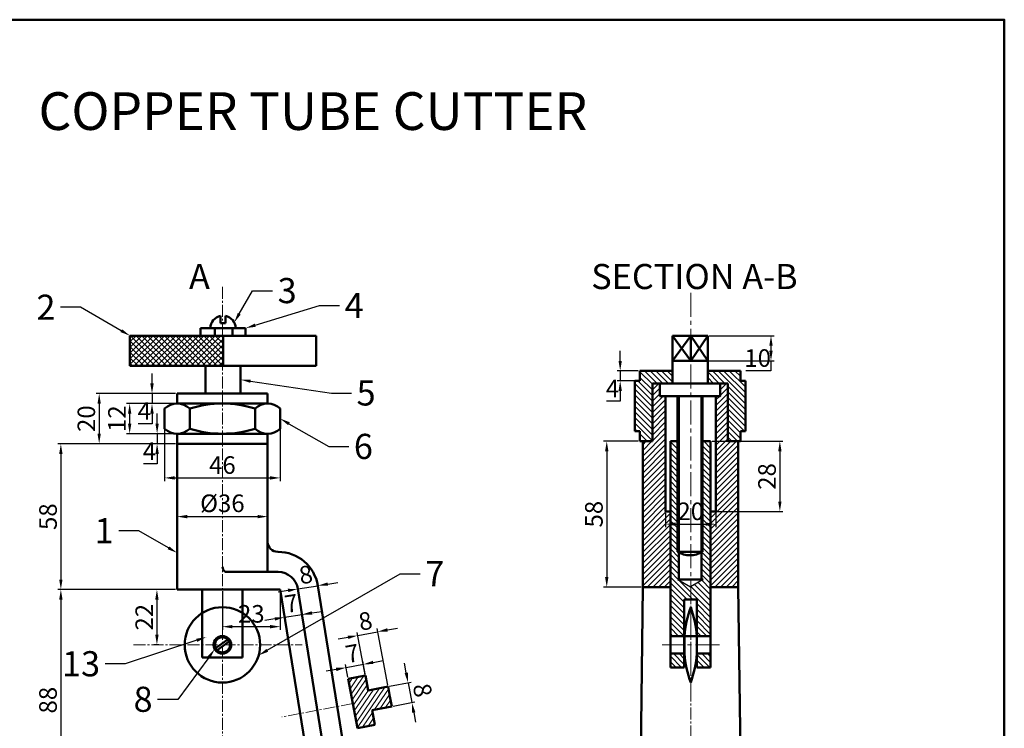
# Model space of a CAD drawing. Units: millimetres. Extents: x 376 to 1043, y -28 to 427.
# Tile 5 of 5: x 651 to 1043, y 145 to 427. Entities that reach past the tile are written whole.
import ezdxf
from ezdxf import colors
from ezdxf.entities.mleader import LeaderData, LeaderLine
from ezdxf.math import Vec2, Vec3

# ---------------------------------------------------------------- set-up
doc = ezdxf.new("R2010")
doc.units = ezdxf.units.MM
doc.header["$LTSCALE"] = 0.5
doc.linetypes.add('CENTER2', pattern=[28.575, 19.05, -3.175, 3.175, -3.175])
doc.linetypes.add('DASHED', pattern=[19.05, 12.7, -6.35])
for name, color, linetype, lineweight in [('M-CNTR', 1, 'CENTER2', 18), ('M-DIMS', 2, 'Continuous', 25), ('M-HATC', 8, 'Continuous', 18), ('M-HIDN', 4, 'DASHED', 25), ('M-OUTL', 7, 'Continuous', 50), ('M-TEXT', 7, 'Continuous', 25)]:
    doc.layers.add(name, color=color, linetype=linetype, lineweight=lineweight)
doc.styles.get("Standard").update_dxf_attribs({"font": 'arial.ttf'})
doc.dimstyles.new('ISO-25', dxfattribs={"dimtxt": 7, "dimasz": 4, "dimexe": 1.25, "dimexo": 0.625, "dimtad": 1, "dimtoh": 1, "dimtxsty": 'Standard', "dimcen": 2.5, "dimadec": 0, "dimazin": 0, "dimtfac": 1, "dimtmove": 0, "dimatfit": 3, "dimfxl": 1, "dimarcsym": 0})
pattern_1 = [(135, (1108.3857, -159.2338), (-1.122532, -1.122532), [])]

# ---------------------------------------------------------------- blocks, each defined once
blk = doc.blocks.new('*U20')
at = {"layer": 'M-CNTR', "color": 0, "transparency": 16777216}
blk.add_line((0, 74.83), (0, -77.3), dxfattribs=at)
blk = doc.blocks.new('*U26')
at = {"layer": 'M-CNTR', "color": 0, "transparency": 16777216}
blk.add_line((6.25, 0), (-16.57, 0), dxfattribs=at)
blk = doc.blocks.new('*D57')
at = {"layer": 'Defpoints', "color": 0, "ltscale": 0.5, "transparency": 16777216}
for p in [(713.94, 278.26), (703.95, 274.26), (713.94, 274.26)]:
    blk.add_point(p, dxfattribs=at)
at = {"layer": 'M-DIMS', "color": 0, "lineweight": -2, "ltscale": 0.5, "transparency": 16777216}
for p, q in [((703.95, 282.26), (703.95, 286.26)), ((713.32, 278.26), (702.7, 278.26)), ((703.95, 278.26), (703.95, 274.26)), ((713.32, 274.26), (702.7, 274.26)), ((703.95, 270.26), (703.95, 266.26)), ((703.95, 266.26), (698.48, 266.26))]:
    blk.add_line(p, q, dxfattribs=at)
at = {"layer": 'M-DIMS', "color": 0, "ltscale": 0.5, "transparency": 16777216}
for points in [[(703.28, 282.26), (704.62, 282.26), (703.95, 278.26)], [(703.28, 270.26), (704.62, 270.26), (703.95, 274.26)]]:
    blk.add_solid(points, dxfattribs=at)
at = {"layer": 'M-DIMS', "color": 0, "ltscale": 0.5, "transparency": 16777216, "insert": (700.9, 270.39), "char_height": 7, "attachment_point": 5}
blk.add_mtext('4', dxfattribs=at)
blk = doc.blocks.new('*D58')
at = {"layer": 'Defpoints', "color": 0, "ltscale": 0.5, "transparency": 16777216}
for p in [(713.94, 274.26), (695.06, 262.26), (713.94, 262.26)]:
    blk.add_point(p, dxfattribs=at)
at = {"layer": 'M-DIMS', "color": 0, "lineweight": -2, "ltscale": 0.5, "transparency": 16777216}
for p, q in [((713.32, 274.26), (693.81, 274.26)), ((695.06, 270.26), (695.06, 266.26)), ((713.32, 262.26), (693.81, 262.26))]:
    blk.add_line(p, q, dxfattribs=at)
at = {"layer": 'M-DIMS', "color": 0, "ltscale": 0.5, "transparency": 16777216}
for points in [[(694.4, 270.26), (695.73, 270.26), (695.06, 274.26)], [(694.4, 266.26), (695.73, 266.26), (695.06, 262.26)]]:
    blk.add_solid(points, dxfattribs=at)
at = {"layer": 'M-DIMS', "color": 0, "ltscale": 0.5, "transparency": 16777216, "insert": (690.92, 268.26), "char_height": 7, "attachment_point": 5, "rotation": 90}
blk.add_mtext('12', dxfattribs=at)
blk = doc.blocks.new('*D59')
at = {"layer": 'Defpoints', "color": 0, "ltscale": 0.5, "transparency": 16777216}
for p in [(713.94, 262.26), (705.98, 258.26), (713.94, 258.26)]:
    blk.add_point(p, dxfattribs=at)
at = {"layer": 'M-DIMS', "color": 0, "lineweight": -2, "ltscale": 0.5, "transparency": 16777216}
for p, q in [((705.98, 266.26), (705.98, 270.26)), ((713.32, 262.26), (704.73, 262.26)), ((705.98, 262.26), (705.98, 258.26)), ((713.32, 258.26), (704.73, 258.26)), ((705.98, 254.26), (705.98, 250.26)), ((705.98, 250.26), (700.52, 250.26))]:
    blk.add_line(p, q, dxfattribs=at)
at = {"layer": 'M-DIMS', "color": 0, "ltscale": 0.5, "transparency": 16777216}
for points in [[(705.32, 266.26), (706.65, 266.26), (705.98, 262.26)], [(705.32, 254.26), (706.65, 254.26), (705.98, 258.26)]]:
    blk.add_solid(points, dxfattribs=at)
at = {"layer": 'M-DIMS', "color": 0, "ltscale": 0.5, "transparency": 16777216, "insert": (702.94, 254.39), "char_height": 7, "attachment_point": 5}
blk.add_mtext('4', dxfattribs=at)
blk = doc.blocks.new('*D60')
at = {"layer": 'Defpoints', "color": 0, "ltscale": 0.5, "transparency": 16777216}
for p in [(713.94, 278.26), (682.94, 258.26), (713.94, 258.26)]:
    blk.add_point(p, dxfattribs=at)
at = {"layer": 'M-DIMS', "color": 0, "lineweight": -2, "ltscale": 0.5, "transparency": 16777216}
for p, q in [((713.32, 278.26), (681.69, 278.26)), ((682.94, 274.26), (682.94, 262.26)), ((713.32, 258.26), (681.69, 258.26))]:
    blk.add_line(p, q, dxfattribs=at)
at = {"layer": 'M-DIMS', "color": 0, "ltscale": 0.5, "transparency": 16777216}
for points in [[(682.27, 274.26), (683.6, 274.26), (682.94, 278.26)], [(682.27, 262.26), (683.6, 262.26), (682.94, 258.26)]]:
    blk.add_solid(points, dxfattribs=at)
at = {"layer": 'M-DIMS', "color": 0, "ltscale": 0.5, "transparency": 16777216, "insert": (678.74, 268.26), "char_height": 7, "attachment_point": 5, "rotation": 90}
blk.add_mtext('20', dxfattribs=at)
blk = doc.blocks.new('*D61')
at = {"layer": 'Defpoints', "color": 0, "ltscale": 0.5, "transparency": 16777216}
for p in [(697.5, 258.26), (667.7, 200.26), (713.94, 200.26)]:
    blk.add_point(p, dxfattribs=at)
at = {"layer": 'M-DIMS', "color": 0, "lineweight": -2, "ltscale": 0.5, "transparency": 16777216}
for p, q in [((696.88, 258.26), (666.45, 258.26)), ((667.7, 254.26), (667.7, 204.26)), ((713.32, 200.26), (666.45, 200.26))]:
    blk.add_line(p, q, dxfattribs=at)
at = {"layer": 'M-DIMS', "color": 0, "ltscale": 0.5, "transparency": 16777216}
for points in [[(667.03, 254.26), (668.37, 254.26), (667.7, 258.26)], [(667.03, 204.26), (668.37, 204.26), (667.7, 200.26)]]:
    blk.add_solid(points, dxfattribs=at)
at = {"layer": 'M-DIMS', "color": 0, "ltscale": 0.5, "transparency": 16777216, "insert": (663.5, 229.26), "char_height": 7, "attachment_point": 5, "rotation": 90}
blk.add_mtext('58', dxfattribs=at)
blk = doc.blocks.new('*D62')
at = {"layer": 'Defpoints', "color": 0, "ltscale": 0.5, "transparency": 16777216}
for p in [(707.25, 200.26), (705.91, 178.26), (707.25, 178.26)]:
    blk.add_point(p, dxfattribs=at)
at = {"layer": 'M-DIMS', "color": 0, "lineweight": -2, "ltscale": 0.5, "transparency": 16777216}
for p, q in [((706.63, 200.26), (704.66, 200.26)), ((705.91, 196.26), (705.91, 182.26)), ((706.63, 178.26), (704.66, 178.26))]:
    blk.add_line(p, q, dxfattribs=at)
at = {"layer": 'M-DIMS', "color": 0, "ltscale": 0.5, "transparency": 16777216}
for points in [[(705.24, 196.26), (706.57, 196.26), (705.91, 200.26)], [(705.24, 182.26), (706.57, 182.26), (705.91, 178.26)]]:
    blk.add_solid(points, dxfattribs=at)
at = {"layer": 'M-DIMS', "color": 0, "ltscale": 0.5, "transparency": 16777216, "insert": (701.77, 189.26), "char_height": 7, "attachment_point": 5, "rotation": 90}
blk.add_mtext('22', dxfattribs=at)
blk = doc.blocks.new('*D63')
at = {"layer": 'Defpoints', "color": 0, "ltscale": 0.5, "transparency": 16777216}
for p in [(689.88, 200.26), (667.7, 112.26), (689.88, 112.26)]:
    blk.add_point(p, dxfattribs=at)
at = {"layer": 'M-DIMS', "color": 0, "lineweight": -2, "ltscale": 0.5, "transparency": 16777216}
for p, q in [((689.26, 200.26), (666.45, 200.26)), ((667.7, 196.26), (667.7, 116.26)), ((689.26, 112.26), (666.45, 112.26))]:
    blk.add_line(p, q, dxfattribs=at)
at = {"layer": 'M-DIMS', "color": 0, "ltscale": 0.5, "transparency": 16777216}
for points in [[(667.03, 196.26), (668.37, 196.26), (667.7, 200.26)], [(667.03, 116.26), (668.37, 116.26), (667.7, 112.26)]]:
    blk.add_solid(points, dxfattribs=at)
at = {"layer": 'M-DIMS', "color": 0, "ltscale": 0.5, "transparency": 16777216, "insert": (663.5, 156.26), "char_height": 7, "attachment_point": 5, "rotation": 90}
blk.add_mtext('88', dxfattribs=at)
blk = doc.blocks.new('*D76')
at = {"layer": 'Defpoints', "color": 0, "ltscale": 0.5, "transparency": 16777216}
for p in [(756.71, 189.23), (763.62, 190.33), (763.62, 190.33)]:
    blk.add_point(p, dxfattribs=at)
at = {"layer": 'M-DIMS', "color": 0, "lineweight": -2, "ltscale": 0.5, "transparency": 16777216}
for p, q in [((752.76, 188.59), (748.81, 187.96)), ((756.61, 189.84), (756.51, 190.46)), ((756.71, 189.23), (763.62, 190.33)), ((763.53, 190.95), (763.43, 191.57)), ((767.57, 190.97), (771.52, 191.6))]:
    blk.add_line(p, q, dxfattribs=at)
at = {"layer": 'M-DIMS', "color": 0, "ltscale": 0.5, "transparency": 16777216}
for points in [[(752.66, 189.25), (752.87, 187.93), (756.71, 189.23)], [(767.47, 191.63), (767.68, 190.31), (763.62, 190.33)]]:
    blk.add_solid(points, dxfattribs=at)
at = {"layer": 'M-DIMS', "color": 0, "ltscale": 0.5, "transparency": 16777216, "insert": (759.52, 193.85), "char_height": 7, "attachment_point": 5, "rotation": 9.1114}
blk.add_mtext('7', dxfattribs=at)
blk = doc.blocks.new('*D77')
at = {"layer": 'Defpoints', "color": 0, "ltscale": 0.5, "transparency": 16777216}
for p in [(761.99, 200.53), (769.89, 201.8), (769.89, 201.8)]:
    blk.add_point(p, dxfattribs=at)
at = {"layer": 'M-DIMS', "color": 0, "lineweight": -2, "ltscale": 0.5, "transparency": 16777216}
for p, q in [((758.04, 199.9), (754.09, 199.26)), ((761.99, 200.53), (769.89, 201.8)), ((762.09, 199.91), (762.19, 199.3)), ((769.99, 201.18), (770.09, 200.56)), ((773.84, 202.43), (777.79, 203.06))]:
    blk.add_line(p, q, dxfattribs=at)
at = {"layer": 'M-DIMS', "color": 0, "ltscale": 0.5, "transparency": 16777216}
for points in [[(757.93, 200.56), (758.15, 199.24), (761.99, 200.53)], [(773.73, 203.09), (773.94, 201.77), (769.89, 201.8)]]:
    blk.add_solid(points, dxfattribs=at)
at = {"layer": 'M-DIMS', "color": 0, "ltscale": 0.5, "transparency": 16777216, "insert": (765.27, 205.31), "char_height": 7, "attachment_point": 5, "rotation": 9.1114}
blk.add_mtext('8', dxfattribs=at)
blk = doc.blocks.new('*D78')
at = {"layer": 'Defpoints', "color": 0, "ltscale": 0.5, "transparency": 16777216}
for p in [(731.94, 200.26), (754.94, 200.26), (731.94, 185.5)]:
    blk.add_point(p, dxfattribs=at)
at = {"layer": 'M-DIMS', "color": 0, "lineweight": -2, "ltscale": 0.5, "transparency": 16777216}
for p, q in [((731.94, 199.64), (731.94, 184.25)), ((754.94, 199.64), (754.94, 184.25)), ((750.94, 185.5), (735.94, 185.5))]:
    blk.add_line(p, q, dxfattribs=at)
at = {"layer": 'M-DIMS', "color": 0, "ltscale": 0.5, "transparency": 16777216}
for points in [[(735.94, 186.17), (735.94, 184.83), (731.94, 185.5)], [(750.94, 186.17), (750.94, 184.83), (754.94, 185.5)]]:
    blk.add_solid(points, dxfattribs=at)
at = {"layer": 'M-DIMS', "color": 0, "ltscale": 0.5, "transparency": 16777216, "insert": (743.44, 189.7), "char_height": 7, "attachment_point": 5}
blk.add_mtext('23', dxfattribs=at)
blk = doc.blocks.new('*D79')
at = {"layer": 'Defpoints', "color": 0, "ltscale": 0.5, "transparency": 16777216}
for p in [(713.94, 229.26), (749.94, 229.29), (749.94, 229.26)]:
    blk.add_point(p, dxfattribs=at)
at = {"layer": 'M-DIMS', "color": 0, "lineweight": -2, "ltscale": 0.5, "transparency": 16777216}
for p, q in [((713.94, 229.89), (713.94, 230.54)), ((717.94, 229.29), (745.94, 229.29)), ((749.94, 229.89), (749.94, 230.54))]:
    blk.add_line(p, q, dxfattribs=at)
at = {"layer": 'M-DIMS', "color": 0, "ltscale": 0.5, "transparency": 16777216}
for points in [[(717.94, 229.96), (717.94, 228.62), (713.94, 229.29)], [(745.94, 229.96), (745.94, 228.62), (749.94, 229.29)]]:
    blk.add_solid(points, dxfattribs=at)
at = {"layer": 'M-DIMS', "color": 0, "ltscale": 0.5, "transparency": 16777216, "insert": (731.94, 233.68), "char_height": 7, "attachment_point": 5}
blk.add_mtext('%%C36', dxfattribs=at)
blk = doc.blocks.new('*D80')
at = {"layer": 'Defpoints', "color": 0, "ltscale": 0.5, "transparency": 16777216}
for p in [(708.94, 268.26), (754.94, 268.26), (754.94, 244.69)]:
    blk.add_point(p, dxfattribs=at)
at = {"layer": 'M-DIMS', "color": 0, "lineweight": -2, "ltscale": 0.5, "transparency": 16777216}
for p, q in [((708.94, 267.64), (708.94, 243.44)), ((754.94, 267.64), (754.94, 243.44)), ((712.94, 244.69), (750.94, 244.69))]:
    blk.add_line(p, q, dxfattribs=at)
at = {"layer": 'M-DIMS', "color": 0, "ltscale": 0.5, "transparency": 16777216}
for points in [[(712.94, 245.35), (712.94, 244.02), (708.94, 244.69)], [(750.94, 245.35), (750.94, 244.02), (754.94, 244.69)]]:
    blk.add_solid(points, dxfattribs=at)
at = {"layer": 'M-DIMS', "color": 0, "ltscale": 0.5, "transparency": 16777216, "insert": (731.94, 248.89), "char_height": 7, "attachment_point": 5}
blk.add_mtext('46', dxfattribs=at)
blk = doc.blocks.new('*D82')
at = {"layer": 'Defpoints', "color": 0, "ltscale": 0.5, "transparency": 16777216}
for p in [(788, 170.53), (781.97, 164.76), (788.85, 166.07)]:
    blk.add_point(p, dxfattribs=at)
at = {"layer": 'M-DIMS', "color": 0, "lineweight": -2, "ltscale": 0.5, "transparency": 16777216}
for p, q in [((777.19, 168.49), (773.26, 167.74)), ((781.85, 165.38), (780.89, 170.46)), ((781.12, 169.23), (788, 170.53)), ((788.73, 166.68), (787.77, 171.76)), ((791.93, 171.28), (795.86, 172.02))]:
    blk.add_line(p, q, dxfattribs=at)
at = {"layer": 'M-DIMS', "color": 0, "ltscale": 0.5, "transparency": 16777216}
for points in [[(777.07, 169.14), (777.32, 167.83), (781.12, 169.23)], [(791.81, 171.93), (792.05, 170.62), (788, 170.53)]]:
    blk.add_solid(points, dxfattribs=at)
at = {"layer": 'M-DIMS', "color": 0, "ltscale": 0.5, "transparency": 16777216, "insert": (783.79, 173.94), "char_height": 7, "attachment_point": 5, "rotation": 10.7228}
blk.add_mtext('7', dxfattribs=at)
blk = doc.blocks.new('*D83')
at = {"layer": 'Defpoints', "color": 0, "ltscale": 0.5, "transparency": 16777216}
for p in [(793.69, 183.49), (797.82, 161.66), (789.96, 160.17)]:
    blk.add_point(p, dxfattribs=at)
at = {"layer": 'M-DIMS', "color": 0, "lineweight": -2, "ltscale": 0.5, "transparency": 16777216}
for p, q in [((797.71, 162.27), (793.46, 184.71)), ((797.62, 184.23), (801.55, 184.97)), ((781.9, 181.25), (777.97, 180.51)), ((789.85, 160.78), (785.6, 183.23)), ((785.83, 182), (793.69, 183.49))]:
    blk.add_line(p, q, dxfattribs=at)
at = {"layer": 'M-DIMS', "color": 0, "ltscale": 0.5, "transparency": 16777216}
for points in [[(797.49, 184.89), (797.74, 183.58), (793.69, 183.49)], [(781.77, 181.91), (782.02, 180.6), (785.83, 182)]]:
    blk.add_solid(points, dxfattribs=at)
at = {"layer": 'M-DIMS', "color": 0, "ltscale": 0.5, "transparency": 16777216, "insert": (788.98, 186.87), "char_height": 7, "attachment_point": 5, "rotation": 10.7228}
blk.add_mtext('8', dxfattribs=at)
blk = doc.blocks.new('*D84')
at = {"layer": 'Defpoints', "color": 0, "ltscale": 0.5, "transparency": 16777216}
for p in [(797.82, 161.66), (799.31, 153.8), (807.29, 155.31)]:
    blk.add_point(p, dxfattribs=at)
at = {"layer": 'M-DIMS', "color": 0, "lineweight": -2, "ltscale": 0.5, "transparency": 16777216}
for p, q in [((805.06, 167.1), (804.32, 171.03)), ((798.44, 161.77), (807.03, 163.4)), ((805.8, 163.17), (807.29, 155.31)), ((799.92, 153.91), (808.52, 155.54)), ((808.04, 151.38), (808.78, 147.45))]:
    blk.add_line(p, q, dxfattribs=at)
at = {"layer": 'M-DIMS', "color": 0, "ltscale": 0.5, "transparency": 16777216}
for points in [[(805.72, 167.22), (804.41, 166.98), (805.8, 163.17)], [(808.69, 151.5), (807.38, 151.26), (807.29, 155.31)]]:
    blk.add_solid(points, dxfattribs=at)
at = {"layer": 'M-DIMS', "color": 0, "ltscale": 0.5, "transparency": 16777216, "insert": (810.67, 160.02), "char_height": 7, "attachment_point": 5, "rotation": 280.7228}
blk.add_mtext('8', dxfattribs=at)
blk = doc.blocks.new('*D88')
at = {"layer": 'Defpoints', "color": 0, "ltscale": 0.5, "transparency": 16777216}
for p in [(908.2, 231.26), (928.2, 231.26), (928.2, 226.29)]:
    blk.add_point(p, dxfattribs=at)
at = {"layer": 'M-DIMS', "color": 0, "lineweight": -2, "ltscale": 0.5, "transparency": 16777216}
for p, q in [((908.2, 230.64), (908.2, 225.04)), ((928.2, 230.64), (928.2, 225.04)), ((912.2, 226.29), (924.2, 226.29))]:
    blk.add_line(p, q, dxfattribs=at)
at = {"layer": 'M-DIMS', "color": 0, "ltscale": 0.5, "transparency": 16777216}
for points in [[(912.2, 226.96), (912.2, 225.62), (908.2, 226.29)], [(924.2, 226.96), (924.2, 225.62), (928.2, 226.29)]]:
    blk.add_solid(points, dxfattribs=at)
at = {"layer": 'M-DIMS', "color": 0, "ltscale": 0.5, "transparency": 16777216, "insert": (918.2, 230.49), "char_height": 7, "attachment_point": 5}
blk.add_mtext('20', dxfattribs=at)
blk = doc.blocks.new('*D89')
at = {"layer": 'Defpoints', "color": 0, "ltscale": 0.5, "transparency": 16777216}
for p in [(897.95, 259.26), (884.8, 201.26), (899.11, 201.26)]:
    blk.add_point(p, dxfattribs=at)
at = {"layer": 'M-DIMS', "color": 0, "lineweight": -2, "ltscale": 0.5, "transparency": 16777216}
for p, q in [((897.32, 259.26), (883.55, 259.26)), ((884.8, 255.26), (884.8, 205.26)), ((898.48, 201.26), (883.55, 201.26))]:
    blk.add_line(p, q, dxfattribs=at)
at = {"layer": 'M-DIMS', "color": 0, "ltscale": 0.5, "transparency": 16777216}
for points in [[(884.13, 255.26), (885.47, 255.26), (884.8, 259.26)], [(884.13, 205.26), (885.47, 205.26), (884.8, 201.26)]]:
    blk.add_solid(points, dxfattribs=at)
at = {"layer": 'M-DIMS', "color": 0, "ltscale": 0.5, "transparency": 16777216, "insert": (880.6, 230.26), "char_height": 7, "attachment_point": 5, "rotation": 90}
blk.add_mtext('58', dxfattribs=at)
blk = doc.blocks.new('*D90')
at = {"layer": 'Defpoints', "color": 0, "ltscale": 0.5, "transparency": 16777216}
for p in [(924.95, 301.26), (924.95, 291.26), (950.12, 291.26)]:
    blk.add_point(p, dxfattribs=at)
at = {"layer": 'M-DIMS', "color": 0, "lineweight": -2, "ltscale": 0.5, "transparency": 16777216}
for p, q in [((925.57, 301.26), (951.37, 301.26)), ((950.12, 297.26), (950.12, 295.26)), ((925.57, 291.26), (951.37, 291.26)), ((950.12, 291.26), (950.12, 287.26)), ((950.12, 287.26), (940.15, 287.26))]:
    blk.add_line(p, q, dxfattribs=at)
at = {"layer": 'M-DIMS', "color": 0, "ltscale": 0.5, "transparency": 16777216}
for points in [[(949.46, 297.26), (950.79, 297.26), (950.12, 301.26)], [(949.46, 295.26), (950.79, 295.26), (950.12, 291.26)]]:
    blk.add_solid(points, dxfattribs=at)
at = {"layer": 'M-DIMS', "color": 0, "ltscale": 0.5, "transparency": 16777216, "insert": (944.83, 291.46), "char_height": 7, "attachment_point": 5}
blk.add_mtext('10', dxfattribs=at)
blk = doc.blocks.new('*D91')
at = {"layer": 'Defpoints', "color": 0, "ltscale": 0.5, "transparency": 16777216}
for p in [(926.11, 259.26), (926.11, 231.26), (953.65, 231.26)]:
    blk.add_point(p, dxfattribs=at)
at = {"layer": 'M-DIMS', "color": 0, "lineweight": -2, "ltscale": 0.5, "transparency": 16777216}
for p, q in [((926.73, 259.26), (954.9, 259.26)), ((953.65, 255.26), (953.65, 235.26)), ((926.73, 231.26), (954.9, 231.26))]:
    blk.add_line(p, q, dxfattribs=at)
at = {"layer": 'M-DIMS', "color": 0, "ltscale": 0.5, "transparency": 16777216}
for points in [[(952.99, 255.26), (954.32, 255.26), (953.65, 259.26)], [(952.99, 235.26), (954.32, 235.26), (953.65, 231.26)]]:
    blk.add_solid(points, dxfattribs=at)
at = {"layer": 'M-DIMS', "color": 0, "ltscale": 0.5, "transparency": 16777216, "insert": (949.45, 245.26), "char_height": 7, "attachment_point": 5, "rotation": 90}
blk.add_mtext('28', dxfattribs=at)
blk = doc.blocks.new('*D92')
at = {"layer": 'Defpoints', "color": 0, "ltscale": 0.5, "transparency": 16777216}
for p in [(897.95, 287.26), (890.15, 283.26), (897.95, 283.26)]:
    blk.add_point(p, dxfattribs=at)
at = {"layer": 'M-DIMS', "color": 0, "lineweight": -2, "ltscale": 0.5, "transparency": 16777216}
for p, q in [((890.15, 291.26), (890.15, 295.26)), ((897.32, 287.26), (888.9, 287.26)), ((890.15, 287.26), (890.15, 283.26)), ((897.32, 283.26), (888.9, 283.26)), ((890.15, 279.26), (890.15, 275.26)), ((890.15, 275.26), (884.69, 275.26))]:
    blk.add_line(p, q, dxfattribs=at)
at = {"layer": 'M-DIMS', "color": 0, "ltscale": 0.5, "transparency": 16777216}
for points in [[(889.49, 291.26), (890.82, 291.26), (890.15, 287.26)], [(889.49, 279.26), (890.82, 279.26), (890.15, 283.26)]]:
    blk.add_solid(points, dxfattribs=at)
at = {"layer": 'M-DIMS', "color": 0, "ltscale": 0.5, "transparency": 16777216, "insert": (887.11, 279.39), "char_height": 7, "attachment_point": 5}
blk.add_mtext('4', dxfattribs=at)

msp = doc.modelspace()

# ---------------------------------------------------------------- hatches: boundary and pattern name
at = {"layer": 'M-HATC', "ltscale": 0.5}
h = msp.add_hatch(dxfattribs=at)
h.set_pattern_fill('ANSI37', color=256, scale=0.5)
h.set_pattern_definition([(45, (907.5903, -133.1619), (-1.122532, 1.122532), []), (135, (907.5903, -133.1619), (-1.122532, -1.122532), [])])
h.paths.add_polyline_path([(732.193, 289.264), (732.193, 301.264), (695.193, 301.264), (695.193, 289.264)])
h = msp.add_hatch(dxfattribs=at)
h.set_pattern_fill('ANSI31', color=256, scale=0.5, angle=90)
h.set_pattern_definition(pattern_1)
h.paths.add_polyline_path([(902.946, 282.264), (905.946, 282.264), (910.946, 282.264), (910.946, 287.264), (897.946, 287.264), (897.946, 283.264), (895.946, 283.264), (895.946, 263.264), (897.946, 263.264), (897.946, 259.264), (902.946, 259.264)])
h.paths.add_polyline_path([(939.946, 283.264), (937.946, 283.264), (937.946, 287.264), (924.946, 287.264), (924.946, 282.264), (929.946, 282.264), (932.946, 282.264), (932.946, 273.535), (932.946, 259.264), (937.946, 259.264), (937.946, 263.264), (939.946, 263.264)])
h = msp.add_hatch(dxfattribs=at)
h.set_pattern_fill('ANSI31', color=256, scale=0.5)
h.set_pattern_definition([(45, (1108.3857, -159.2338), (-1.122532, 1.122532), [])])
h.paths.add_polyline_path([(899.107, 201.264), (910.107, 201.264), (910.107, 231.264), (908.196, 231.264), (908.196, 277.264), (905.946, 277.264), (905.946, 282.264), (902.946, 282.264), (902.946, 259.264), (899.107, 259.264)])
h.paths.add_polyline_path([(937.107, 259.264), (932.946, 259.264), (932.946, 273.535), (932.946, 282.264), (929.946, 282.264), (929.946, 277.264), (928.196, 277.264), (928.196, 231.264), (926.107, 231.264), (926.107, 201.264), (937.107, 201.264)])
h = msp.add_hatch(dxfattribs=at)
h.set_pattern_fill('ANSI31', color=256, scale=0.5, angle=90)
h.set_pattern_definition(pattern_1)
h.paths.add_polyline_path([(926.107, 259.264), (922.946, 259.264), (922.946, 215.264, -0.0142093), (922.446, 214.994), (922.446, 204.264), (923.107, 204.264), (918.107, 201.378), (913.107, 204.264), (913.446, 204.264), (913.446, 214.994, -0.0142093), (912.946, 215.264), (912.946, 259.264), (910.107, 259.264), (910.107, 181.764), (915.607, 181.764), (915.607, 196.264), (920.607, 196.264), (920.607, 182.699, -0.0051135), (920.696, 181.764), (926.107, 181.764)])
h = msp.add_hatch(dxfattribs=at)
h.set_pattern_fill('ANSI31', color=256, scale=0.5, angle=90)
h.set_pattern_definition(pattern_1)
h.paths.add_polyline_path([(915.607, 174.764), (910.107, 174.764), (910.107, 169.264), (915.607, 169.264)])
h.paths.add_polyline_path([(926.107, 174.764), (920.696, 174.764, -0.0051135), (920.607, 173.83), (920.607, 169.264), (926.107, 169.264)])
h = msp.add_hatch(dxfattribs=at)
h.set_pattern_fill('ANSI31', color=256, scale=0.5, angle=10.7228)
h.set_pattern_definition([(55.7228, (1132.0873, -118.6822), (-1.311787, 0.8940756), [])])
h.paths.add_polyline_path([(799.31, 153.798), (798.566, 157.728), (797.822, 161.659), (789.962, 160.17), (788.845, 166.065), (781.967, 164.763), (785.689, 145.112), (792.566, 146.415), (791.45, 152.31)])

# ---------------------------------------------------------------- linework, layer by layer
at = {"layer": 'M-CNTR', "ltscale": 0.5}
for p, q in [((731.943, 320.737), (731.943, -3.612)), ((918.196, 160.434), (918.196, 196.785)), ((696.645, 178.264), (763.736, 178.264)), ((918.196, 160.434), (918.196, 11.662)), ((783.828, 154.938), (755.538, 149.58))]:
    msp.add_line(p, q, dxfattribs=at)
at = {"layer": 'M-HIDN'}
for p, q in [((913.107, 215.264), (913.107, 215.174)), ((922.607, 215.264), (922.607, 215.077)), ((913.107, 204.264), (918.107, 201.378)), ((923.107, 204.264), (918.107, 201.378))]:
    msp.add_line(p, q, dxfattribs=at)
at = {"layer": 'M-OUTL'}
for p, q in [((731.193, 306.264), (731.193, 309.163)), ((732.193, 306.264), (731.193, 306.264)), ((732.193, 306.264), (733.193, 306.264)), ((733.193, 306.264), (733.193, 309.163)), ((741.193, 304.264), (723.193, 304.264)), ((723.193, 304.264), (723.193, 301.264)), ((727.193, 304.264), (737.193, 304.264)), ((728.935, 304.264), (728.935, 301.264)), ((735.998, 304.264), (735.998, 301.264)), ((741.193, 301.264), (741.193, 304.264)), ((769.193, 301.264), (695.193, 301.264)), ((695.193, 301.264), (695.193, 289.264)), ((723.193, 301.264), (741.193, 301.264)), ((732.193, 301.264), (732.193, 289.264)), ((769.193, 289.264), (769.193, 301.264)), ((910.946, 301.264), (924.946, 301.264)), ((910.946, 282.264), (910.946, 301.264)), ((924.946, 301.264), (924.946, 282.264)), ((695.193, 289.264), (769.193, 289.264)), ((713.943, 278.264), (724.943, 278.264)), ((713.943, 274.264), (713.943, 278.264)), ((724.943, 278.264), (738.943, 278.264)), ((738.943, 278.264), (749.943, 278.264)), ((749.943, 278.264), (749.943, 274.264)), ((749.943, 274.264), (713.943, 274.264)), ((912.946, 277.264), (912.946, 215.264)), ((913.446, 277.264), (913.446, 204.264)), ((922.446, 277.264), (922.446, 204.264)), ((922.946, 277.264), (922.946, 215.264)), ((910.107, 259.264), (912.946, 259.264)), ((910.107, 169.264), (910.107, 259.264)), ((922.946, 259.264), (926.107, 259.264)), ((926.107, 259.264), (926.107, 169.264)), ((912.946, 215.264), (922.946, 215.264)), ((915.607, 181.764), (910.107, 181.764)), ((926.107, 181.764), (920.607, 181.764)), ((915.607, 174.764), (910.107, 174.764)), ((926.107, 174.764), (920.607, 174.764)), ((915.607, 169.264), (910.107, 169.264)), ((926.107, 169.264), (920.607, 169.264))]:
    msp.add_line(p, q, dxfattribs=at)
at = {"layer": 'M-OUTL', "ltscale": 0.5}
for p, q in [((910.946, 301.264), (924.946, 301.264)), ((918.196, 291.264), (910.946, 301.264)), ((910.946, 291.264), (918.196, 301.264)), ((918.196, 301.264), (918.196, 291.264)), ((918.196, 291.264), (924.946, 301.264)), ((924.946, 291.264), (918.196, 301.264)), ((910.946, 291.264), (924.946, 291.264)), ((725.193, 289.264), (739.193, 289.264)), ((725.193, 278.264), (725.193, 289.264)), ((739.193, 289.264), (739.193, 278.264)), ((910.946, 287.264), (897.946, 287.264)), ((897.946, 287.264), (897.946, 283.264)), ((924.946, 287.264), (937.946, 287.264)), ((937.946, 287.264), (937.946, 283.264)), ((897.946, 283.264), (895.946, 283.264)), ((895.946, 283.264), (895.946, 263.264)), ((905.946, 282.264), (902.946, 282.264)), ((902.946, 282.264), (902.946, 259.264)), ((929.946, 282.264), (932.946, 282.264)), ((932.946, 282.264), (932.946, 273.535)), ((937.946, 283.264), (939.946, 283.264)), ((939.946, 283.264), (939.946, 263.264)), ((739.193, 278.264), (725.193, 278.264)), ((749.943, 274.264), (713.943, 274.264)), ((908.196, 277.264), (908.196, 231.264)), ((928.196, 277.264), (928.196, 231.264)), ((708.943, 272.264), (708.943, 264.264)), ((718.943, 272.264), (718.943, 264.264)), ((744.943, 272.264), (744.943, 264.264)), ((754.943, 264.264), (754.943, 272.264)), ((932.946, 259.264), (932.946, 273.535)), ((895.946, 263.264), (897.946, 263.264)), ((897.946, 263.264), (897.946, 259.264)), ((939.946, 263.264), (937.946, 263.264)), ((937.946, 263.264), (937.946, 259.264)), ((713.943, 262.264), (749.943, 262.264)), ((713.943, 262.264), (713.943, 258.264)), ((749.943, 258.264), (749.943, 262.264)), ((897.946, 259.264), (902.946, 259.264)), ((899.107, 201.264), (899.107, 259.264)), ((937.946, 259.264), (932.946, 259.264)), ((937.107, 201.264), (937.107, 259.264)), ((713.943, 258.264), (749.943, 258.264)), ((713.943, 258.264), (713.943, 200.264)), ((749.943, 207.264), (749.943, 258.264)), ((910.107, 231.264), (908.196, 231.264)), ((928.196, 231.264), (926.107, 231.264)), ((753.943, 215.264), (754.09, 215.264)), ((913.107, 204.264), (923.107, 204.264)), ((713.943, 200.264), (749.943, 200.264)), ((723.943, 173.264), (723.943, 200.264)), ((739.943, 200.264), (739.943, 173.264)), ((749.943, 200.264), (754.943, 200.264)), ((754.943, 200.264), (767.452, 122.264)), ((899.107, 201.264), (897.774, 85.565)), ((899.107, 201.264), (910.107, 201.264)), ((910.107, 201.264), (899.107, 201.264)), ((937.107, 201.264), (926.107, 201.264)), ((937.107, 201.264), (938.703, 85.559)), ((920.607, 196.264), (915.607, 196.264)), ((915.607, 196.264), (915.607, 169.264)), ((920.607, 169.264), (920.607, 196.264)), ((729.251, 176.939), (734.049, 180.4)), ((915.696, 178.264), (915.696, 181.764)), ((915.696, 181.764), (920.696, 181.764)), ((920.696, 181.764), (920.696, 174.764)), ((729.836, 176.128), (734.634, 179.589)), ((915.696, 174.764), (915.696, 178.264)), ((739.943, 173.264), (723.943, 173.264)), ((920.696, 174.764), (920.607, 174.764)), ((788.845, 166.065), (781.967, 164.763)), ((781.967, 164.763), (785.689, 145.112)), ((789.962, 160.17), (788.845, 166.065)), ((797.822, 161.659), (789.962, 160.17)), ((798.566, 157.728), (797.822, 161.659)), ((798.566, 157.728), (799.31, 153.798)), ((799.31, 153.798), (791.45, 152.31)), ((792.566, 146.415), (791.45, 152.31)), ((785.689, 145.112), (792.566, 146.415))]:
    msp.add_line(p, q, dxfattribs=at)
msp.add_lwpolyline([(376.448, 426.986), (1042.916, 426.986), (1042.916, -28.377), (376.448, -28.377)], close=True, dxfattribs=at)
at = {"layer": 'M-OUTL'}
msp.add_lwpolyline([(929.946, 282.264), (929.946, 277.264), (905.946, 277.264), (905.946, 282.264), (910.946, 282.264), (924.946, 282.264)], close=True, dxfattribs=at)
at = {"layer": 'M-OUTL', "ltscale": 0.5}
for points in [[(753.943, 215.264), (754.09, 215.264, -0.3683676), (769.888, 201.798), (787.369, 92.798, -0.4615956), (771.571, 74.264)], [(732.986, 207.264), (754.09, 207.264, -0.3683676), (761.989, 200.531), (779.47, 91.531, -0.4615956), (771.571, 82.264)]]:
    msp.add_lwpolyline(points, format="xyb", dxfattribs=at)
for radius in [15, 3.5, 3]:
    msp.add_circle((731.943, 178.264), radius, dxfattribs=at)
at = {"layer": 'M-OUTL'}
for centre, radius, start, end in [((732.193, 304.264), 5, 101.53696, 180), ((732.193, 304.264), 5, 0, 78.46304), ((917.946, 223.925), 10, 240, 300)]:
    msp.add_arc(centre, radius, start, end, dxfattribs=at)
at = {"layer": 'M-OUTL', "ltscale": 0.5}
for centre, radius, start, end in [((713.943, 267.014), 7.25, 46.39718, 133.60282), ((731.943, 231.014), 43.25, 72.50768, 107.49232), ((749.943, 267.014), 7.25, 46.39718, 133.60282), ((713.943, 269.514), 7.25, 226.39718, 313.60282), ((731.943, 305.514), 43.25, 252.50768, 287.49232), ((749.943, 269.514), 7.25, 226.39718, 313.60282), ((753.943, 219.264), 4, 180, 270), ((735.184, 209.669), 3.257, 185.67533, 227.56889), ((961.437, 177.842), 45.908, 160.37106, 175.09939), ((874.956, 177.842), 45.908, 4.90061, 19.62894), ((961.437, 178.686), 45.908, 184.90061, 199.62894), ((874.956, 178.686), 45.908, 340.37106, 355.09939)]:
    msp.add_arc(centre, radius, start, end, dxfattribs=at)

# ---------------------------------------------------------------- block references
at = {"layer": 'M-CNTR'}
for name, p in [('*U20', (918.196, 243.514)), ('*U26', (923.357, 178.264))]:
    msp.add_blockref(name, p, dxfattribs=at)

# ---------------------------------------------------------------- texts
at = {"layer": 'M-TEXT', "ltscale": 0.5, "attachment_point": 1}
for s, width, insert, char_height in [('COPPER TUBE CUTTER', 245.48777, (658.822, 398.121), 15), ('A', 13.27748, (718.665, 329.809), 10), ('SECTION A-B', 96.27488, (878.633, 329.809), 10)]:
    msp.add_mtext_dynamic_manual_height_columns(s, width=width, gutter_width=12.5, heights=[0], dxfattribs=dict(at, insert=insert, char_height=char_height))

# ---------------------------------------------------------------- dimensions: what is measured, and where the dimension line sits
at = {"layer": 'M-DIMS', "ltscale": 0.5}
for base, p1, p2, picture, middle in [((950.123, 291.264), (924.946, 301.264), (924.946, 291.264), '*D90', (944.825, 291.463)), ((890.154, 283.264), (897.946, 287.264), (897.946, 283.264), '*D92', (887.109, 279.389)), ((703.949, 274.264), (713.943, 278.264), (713.943, 274.264), '*D57', (700.903, 270.389)), ((682.937, 258.264), (713.943, 278.264), (713.943, 258.264), '*D60', (678.738, 268.264)), ((695.064, 262.264), (713.943, 274.264), (713.943, 262.264), '*D58', (690.925, 268.264)), ((705.984, 258.264), (713.943, 262.264), (713.943, 258.264), '*D59', (702.938, 254.389)), ((884.8, 201.264), (897.946, 259.264), (899.107, 201.264), '*D89', (880.601, 230.264)), ((953.653, 231.264), (926.107, 259.264), (926.107, 231.264), '*D91', (949.454, 245.264)), ((667.699, 200.264), (697.502, 258.264), (713.943, 200.264), '*D61', (663.5, 229.264)), ((667.699, 112.264), (689.883, 200.264), (689.883, 112.264), '*D63', (663.5, 156.264)), ((705.907, 178.264), (707.25, 200.264), (707.25, 178.264), '*D62', (701.767, 189.264))]:
    dim = msp.add_linear_dim(base=base, p1=p1, p2=p2, angle=90, dimstyle='ISO-25', override={"dimclrd": 0, "dimclre": 0, "dimclrt": 0}, dxfattribs=at)
    dim.commit()
    dim.dimension.update_dxf_attribs({"geometry": picture, "text_midpoint": middle})
for base, p1, p2, picture, middle in [((754.943, 244.688), (708.943, 268.264), (754.943, 268.264), '*D80', (731.943, 248.887)), ((928.196, 226.291), (908.196, 231.264), (928.196, 231.264), '*D88', (918.196, 230.49))]:
    dim = msp.add_linear_dim(base=base, p1=p1, p2=p2, dimstyle='ISO-25', override={"dimclrd": 0, "dimclre": 0, "dimclrt": 0}, dxfattribs=at)
    dim.commit()
    dim.dimension.update_dxf_attribs({"geometry": picture, "text_midpoint": middle})
dim = msp.add_linear_dim(base=(749.943, 229.289), p1=(713.943, 229.264), p2=(749.943, 229.264), text='%%C<>', dimstyle='ISO-25', override={"dimclrd": 0, "dimclre": 0, "dimclrt": 0}, dxfattribs=at)
dim.commit()
dim.dimension.update_dxf_attribs({"geometry": '*D79', "text_midpoint": (731.943, 233.684)})
for p1, p2, distance, picture, middle in [((761.989, 200.531), (769.888, 201.798), 0, '*D77', (765.274, 205.311)), ((754.943, 200.264), (731.943, 200.264), 14.763, '*D78', (743.443, 189.703)), ((756.713, 189.226), (763.624, 190.335), 0, '*D76', (759.515, 193.853)), ((781.967, 164.763), (788.845, 166.065), 4.548, '*D82', (783.793, 173.935)), ((797.822, 161.659), (799.31, 153.798), 8.125, '*D84', (810.675, 160.021))]:
    dim = msp.add_aligned_dim(p1=p1, p2=p2, distance=distance, dimstyle='ISO-25', override={"dimclrd": 0, "dimclre": 0, "dimclrt": 0}, dxfattribs=at)
    dim.commit()
    dim.dimension.update_dxf_attribs({"geometry": picture, "text_midpoint": middle})
dim = msp.add_linear_dim(base=(793.688, 183.486), p1=(789.962, 160.17), p2=(797.822, 161.659), angle=10.7228, dimstyle='ISO-25', override={"dimclrd": 0, "dimclre": 0, "dimclrt": 0}, dxfattribs=at)
dim.commit()
dim.dimension.update_dxf_attribs({"geometry": '*D83', "text_midpoint": (789.758, 182.742), "dimtype": 161})

# ---------------------------------------------------------------- leaders
ml = msp.add_multileader_mtext('Standard', dxfattribs=at)
ml.set_content('3', color=256)
ml.set_leader_properties()
ml.build(insert=Vec2(0, 0))
ctx = ml.context
ctx.base_point, ctx.char_height, ctx.plane_origin = Vec3(751.921, 319.121), 10, Vec3(736.651, 306.528)
notes = []
notes.append((ctx, [(0, (1, 1, 0), (743.921, 319.121), (1, 0), 8, [(0, [(736.651, 306.528)], 0, [])])]))
ctx.mtext.insert, ctx.mtext.flow_direction = Vec3(753.921, 324.21), 5
ml = msp.add_multileader_mtext('Standard', dxfattribs=at)
ml.set_content('2', color=256)
ml.set_leader_properties()
ml.build(insert=Vec2(0, 0))
ctx = ml.context
ctx.base_point, ctx.char_height, ctx.plane_origin = Vec3(656.941, 312.596), 10, Vec3(695.193, 301.264)
ctx.text_align_type = 2
notes.append((ctx, [(0, (1, 1, 0), (675.565, 312.596), (-1, 0), 8, [(0, [(695.193, 301.264)], 0, [])])]))
ctx.mtext.insert, ctx.mtext.alignment, ctx.mtext.flow_direction = Vec3(665.565, 317.596), 3, 5
ml = msp.add_multileader_mtext('Standard', dxfattribs=at)
ml.set_content('4', color=256)
ml.set_leader_properties()
ml.build(insert=Vec2(0, 0))
ctx = ml.context
ctx.base_point, ctx.char_height, ctx.plane_origin = Vec3(778.569, 313.286), 10, Vec3(741.193, 304.264)
notes.append((ctx, [(0, (1, 1, 0), (770.569, 313.286), (1, 0), 8, [(0, [(741.193, 304.264)], 0, [])])]))
ctx.mtext.insert, ctx.mtext.flow_direction = Vec3(780.569, 318.286), 5
ml = msp.add_multileader_mtext('Standard', dxfattribs=at)
ml.set_content('5', color=256)
ml.set_leader_properties()
ml.build(insert=Vec2(0, 0))
ctx = ml.context
ctx.base_point, ctx.char_height, ctx.plane_origin = Vec3(783.297, 278.408), 10, Vec3(739.193, 283.764)
notes.append((ctx, [(0, (1, 1, 0), (775.297, 278.408), (1, 0), 8, [(0, [(739.193, 283.764)], 0, [])])]))
ctx.mtext.insert, ctx.mtext.flow_direction = Vec3(785.297, 283.493), 5
ml = msp.add_multileader_mtext('Standard', dxfattribs=at)
ml.set_content('6', color=256)
ml.set_leader_properties()
ml.build(insert=Vec2(0, 0))
ctx = ml.context
ctx.base_point, ctx.char_height, ctx.plane_origin = Vec3(782.222, 257.133), 10, Vec3(754.943, 268.264)
notes.append((ctx, [(0, (1, 1, 0), (774.222, 257.133), (1, 0), 8, [(0, [(754.943, 268.264)], 0, [])])]))
ctx.mtext.insert, ctx.mtext.flow_direction = Vec3(784.222, 262.218), 5
ml = msp.add_multileader_mtext('Standard', dxfattribs=at)
ml.set_content('1', color=256)
ml.set_leader_properties()
ml.build(insert=Vec2(0, 0))
ctx = ml.context
ctx.base_point, ctx.char_height, ctx.plane_origin = Vec3(683.024, 223.669), 10, Vec3(713.943, 214.873)
ctx.text_align_type = 2
notes.append((ctx, [(0, (1, 1, 0), (698.708, 223.669), (-1, 0), 8, [(0, [(713.943, 214.873)], 0, [])])]))
ctx.mtext.insert, ctx.mtext.alignment, ctx.mtext.flow_direction = Vec3(688.708, 228.669), 3, 5
ml = msp.add_multileader_mtext('Standard', dxfattribs=at)
ml.set_content('7', color=256)
ml.set_leader_properties()
ml.build(insert=Vec2(0, 0))
ctx = ml.context
ctx.base_point, ctx.char_height, ctx.plane_origin = Vec3(810.64, 206.586), 10, Vec3(746.349, 174.087)
notes.append((ctx, [(0, (1, 1, 0), (802.64, 206.586), (1, 0), 8, [(0, [(746.349, 174.087)], 0, [])])]))
ctx.mtext.insert, ctx.mtext.flow_direction = Vec3(812.64, 211.586), 5
ml = msp.add_multileader_mtext('Standard', dxfattribs=at)
ml.set_content('13', color=256)
ml.set_leader_properties()
ml.build(insert=Vec2(0, 0))
ctx = ml.context
ctx.base_point, ctx.char_height, ctx.plane_origin = Vec3(667.921, 170.658), 10, Vec3(725.543, 181.348)
ctx.text_align_type = 2
notes.append((ctx, [(0, (1, 1, 0), (693.305, 170.658), (-1, 0), 8, [(0, [(725.543, 181.348)], 0, [])])]))
ctx.mtext.insert, ctx.mtext.alignment, ctx.mtext.flow_direction = Vec3(683.305, 175.747), 3, 5
ml = msp.add_multileader_mtext('Standard', dxfattribs=at)
ml.set_content('8', color=256)
ml.set_leader_properties()
ml.build(insert=Vec2(0, 0))
ctx = ml.context
ctx.base_point, ctx.char_height, ctx.plane_origin = Vec3(695.595, 156.526), 10, Vec3(728.911, 176.514)
ctx.text_align_type = 2
notes.append((ctx, [(0, (1, 1, 0), (714.184, 156.526), (-1, 0), 8, [(0, [(728.911, 176.514)], 0, [])])]))
ctx.mtext.insert, ctx.mtext.alignment, ctx.mtext.flow_direction = Vec3(704.184, 161.611), 3, 5
for ctx, leaders in notes:
    for number, flags, end, landing, length, lines in leaders:
        leader = LeaderData()
        leader.index, (leader.has_last_leader_line, leader.has_dogleg_vector, leader.attachment_direction) = number, flags
        leader.last_leader_point, leader.dogleg_vector, leader.dogleg_length = Vec3(end), Vec3(landing), length
        for number, points, colour, breaks in lines:
            line = LeaderLine()
            line.index, line.vertices, line.color, line.breaks = number, Vec3.list(points), colors.encode_raw_color(colour), breaks
            leader.lines.append(line)
        ctx.leaders.append(leader)

doc.saveas('drawing.dxf')
